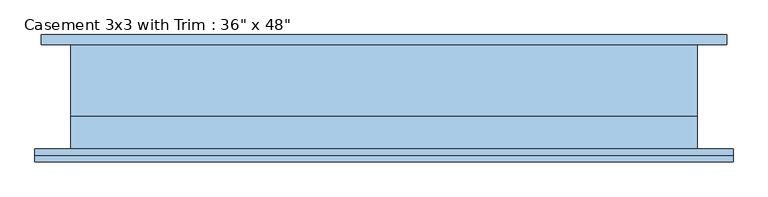
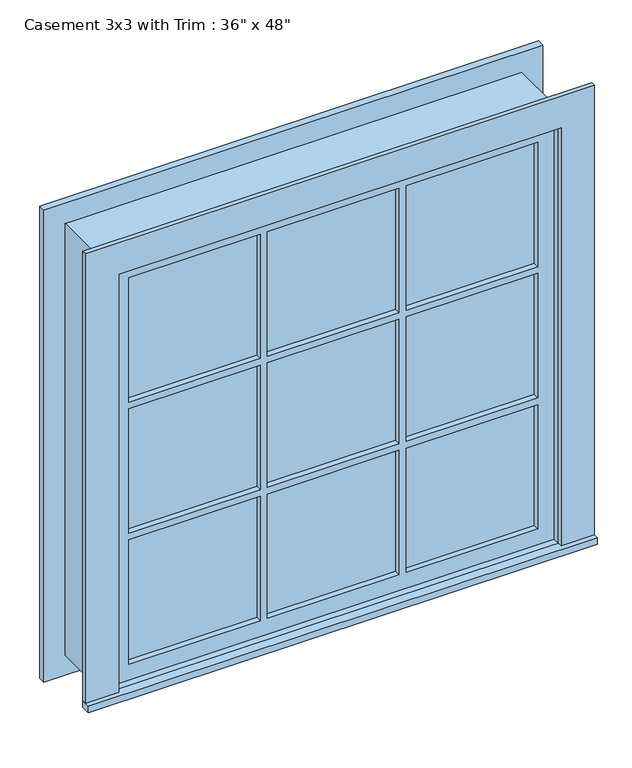
"""IFC4 building model written with IfcOpenShell, lengths in millimetres: window geometry."""

from ifc_helpers import new_model, si_unit, frame, origin, place, context, project, spatial, polyline, outline, extrude, source, transform, mapped, element, save


def window_791d807c(model_context):
    return source(origin(), model_context, "Body", "SweptSolid", [
        extrude(outline(polyline([(-679.45, -127.0), (-679.45, -101.6), (679.45, -101.6), (679.45, -127.0), (-679.45, -127.0)])), frame((0.0, 0.0, 914.4), z_axis=(0.0, 0.0, 1.0), x_axis=(1.0, 0.0, 0.0)), (0.0, 0.0, 1.0), 19.05),
        extrude(outline(polyline([(2114.55, -590.55), (2114.55, 590.55), (933.45, 590.55), (933.45, 679.45), (2203.45, 679.45), (2203.45, -679.45), (933.45, -679.45), (933.45, -590.55), (2114.55, -590.55)])), frame((0.0, -114.3, 0.0), z_axis=(0.0, 1.0, 0.0), x_axis=(0.0, 0.0, 1.0)), (0.0, 0.0, 1.0), 12.7),
        extrude(outline(polyline([(194.7333333, -66.675), (194.7333333, -53.975), (546.1, -53.975), (546.1, -66.675), (194.7333333, -66.675)])), frame((0.0, 0.0, 1718.7333333), z_axis=(0.0, 0.0, 1.0), x_axis=(1.0, 0.0, 0.0)), (0.0, 0.0, 1.0), 351.3666667),
        extrude(outline(polyline([(-175.6833333, -66.675), (-175.6833333, -53.975), (175.6833333, -53.975), (175.6833333, -66.675), (-175.6833333, -66.675)])), frame((0.0, 0.0, 1718.7333333), z_axis=(0.0, 0.0, 1.0), x_axis=(1.0, 0.0, 0.0)), (0.0, 0.0, 1.0), 351.3666667),
        extrude(outline(polyline([(-546.1, -66.675), (-546.1, -53.975), (-194.7333333, -53.975), (-194.7333333, -66.675), (-546.1, -66.675)])), frame((0.0, 0.0, 1718.7333333), z_axis=(0.0, 0.0, 1.0), x_axis=(1.0, 0.0, 0.0)), (0.0, 0.0, 1.0), 351.3666667),
        extrude(outline(polyline([(-546.1, -66.675), (-546.1, -53.975), (-194.7333333, -53.975), (-194.7333333, -66.675), (-546.1, -66.675)])), frame((0.0, 0.0, 1348.3166667), z_axis=(0.0, 0.0, 1.0), x_axis=(1.0, 0.0, 0.0)), (0.0, 0.0, 1.0), 351.3666667),
        extrude(outline(polyline([(-175.6833333, -66.675), (-175.6833333, -53.975), (175.6833333, -53.975), (175.6833333, -66.675), (-175.6833333, -66.675)])), frame((0.0, 0.0, 1348.3166667), z_axis=(0.0, 0.0, 1.0), x_axis=(1.0, 0.0, 0.0)), (0.0, 0.0, 1.0), 351.3666667),
        extrude(outline(polyline([(194.7333333, -66.675), (194.7333333, -53.975), (546.1, -53.975), (546.1, -66.675), (194.7333333, -66.675)])), frame((0.0, 0.0, 1348.3166667), z_axis=(0.0, 0.0, 1.0), x_axis=(1.0, 0.0, 0.0)), (0.0, 0.0, 1.0), 351.3666667),
        extrude(outline(polyline([(194.7333333, -66.675), (194.7333333, -53.975), (546.1, -53.975), (546.1, -66.675), (194.7333333, -66.675)])), frame((0.0, 0.0, 977.9), z_axis=(0.0, 0.0, 1.0), x_axis=(1.0, 0.0, 0.0)), (0.0, 0.0, 1.0), 351.3666667),
        extrude(outline(polyline([(-175.6833333, -66.675), (-175.6833333, -53.975), (175.6833333, -53.975), (175.6833333, -66.675), (-175.6833333, -66.675)])), frame((0.0, 0.0, 977.9), z_axis=(0.0, 0.0, 1.0), x_axis=(1.0, 0.0, 0.0)), (0.0, 0.0, 1.0), 351.3666667),
        extrude(outline(polyline([(-546.1, -66.675), (-546.1, -53.975), (-194.7333333, -53.975), (-194.7333333, -66.675), (-546.1, -66.675)])), frame((0.0, 0.0, 977.9), z_axis=(0.0, 0.0, 1.0), x_axis=(1.0, 0.0, 0.0)), (0.0, 0.0, 1.0), 351.3666667),
        extrude(outline(polyline([(2190.75, 666.75), (2190.75, -666.75), (857.25, -666.75), (857.25, 666.75), (2190.75, 666.75)]), holes=[polyline([(2101.85, 577.85), (946.15, 577.85), (946.15, -577.85), (2101.85, -577.85), (2101.85, 577.85)])]), frame((0.0, 101.6, 0.0), z_axis=(0.0, 1.0, 0.0), x_axis=(0.0, 0.0, 1.0)), (0.0, 0.0, 1.0), 19.05),
        extrude(outline(polyline([(2114.55, -590.55), (933.45, -590.55), (933.45, 590.55), (2114.55, 590.55), (2114.55, -590.55)]), holes=[polyline([(2070.1, -194.7333333), (1718.7333333, -194.7333333), (1718.7333333, -546.1), (2070.1, -546.1), (2070.1, -194.7333333)]), polyline([(1699.6833333, -194.7333333), (1348.3166667, -194.7333333), (1348.3166667, -546.1), (1699.6833333, -546.1), (1699.6833333, -194.7333333)]), polyline([(1329.2666667, -194.7333333), (977.9, -194.7333333), (977.9, -546.1), (1329.2666667, -546.1), (1329.2666667, -194.7333333)]), polyline([(2070.1, 175.6833333), (1718.7333333, 175.6833333), (1718.7333333, -175.6833333), (2070.1, -175.6833333), (2070.1, 175.6833333)]), polyline([(1699.6833333, 175.6833333), (1348.3166667, 175.6833333), (1348.3166667, -175.6833333), (1699.6833333, -175.6833333), (1699.6833333, 175.6833333)]), polyline([(1329.2666667, 175.6833333), (977.9, 175.6833333), (977.9, -175.6833333), (1329.2666667, -175.6833333), (1329.2666667, 175.6833333)]), polyline([(2070.1, 546.1), (1718.7333333, 546.1), (1718.7333333, 194.7333333), (2070.1, 194.7333333), (2070.1, 546.1)]), polyline([(1699.6833333, 546.1), (1348.3166667, 546.1), (1348.3166667, 194.7333333), (1699.6833333, 194.7333333), (1699.6833333, 546.1)]), polyline([(1329.2666667, 546.1), (977.9, 546.1), (977.9, 194.7333333), (1329.2666667, 194.7333333), (1329.2666667, 546.1)])]), frame((0.0, -82.55, 0.0), z_axis=(0.0, 1.0, 0.0), x_axis=(0.0, 0.0, 1.0)), (0.0, 0.0, 1.0), 44.45),
        extrude(outline(polyline([(2133.6, -609.6), (914.4, -609.6), (914.4, 609.6), (2133.6, 609.6), (2133.6, -609.6)]), holes=[polyline([(2101.85, -577.85), (2101.85, 577.85), (946.15, 577.85), (946.15, -577.85), (2101.85, -577.85)])]), frame((0.0, -38.1, 0.0), z_axis=(0.0, 1.0, 0.0), x_axis=(0.0, 0.0, 1.0)), (0.0, 0.0, 1.0), 139.7),
        extrude(outline(polyline([(2133.6, 609.6), (2133.6, -609.6), (914.4, -609.6), (914.4, 609.6), (2133.6, 609.6)]), holes=[polyline([(2114.55, 590.55), (933.45, 590.55), (933.45, -590.55), (2114.55, -590.55), (2114.55, 590.55)])]), frame((0.0, -101.6, 0.0), z_axis=(0.0, 1.0, 0.0), x_axis=(0.0, 0.0, 1.0)), (0.0, 0.0, 1.0), 63.5),
    ])


if __name__ == "__main__":
    model = new_model("IFC4")
    model_context = context("Model", 3, world=origin())
    ifc_project = project(units=[si_unit("LENGTHUNIT", "METRE", prefix="MILLI")], contexts=[model_context])
    site = spatial("IfcSite", under=ifc_project)
    building = spatial("IfcBuilding", under=site)
    placement = place(None, origin())
    window_shape = window_791d807c(model_context)
    element("IfcWindow", 1, ObjectType="Casement 3x3 with Trim : 36\" x 48\"", at=placement, inside=building, context=model_context, shape_type="MappedRepresentation", body=[
        mapped(window_shape, transform((0.0, 0.0, 0.0), x_axis=(1.0, 0.0, 0.0), y_axis=(0.0, 1.0, 0.0), z_axis=(0.0, 0.0, 1.0))),
    ])
    save(model, "model.ifc")

# Revit data of these elements
# Type "Casement 3x3 with Trim : 36\" x 48\""
#   Type Mark = "10"
#   Construction Type Id = "GSP4R"
#   Assembly Code = "B2020100"
#   Analytic Construction = "1/8 in Pilkington single glazing"
#   Visual Light Transmittance = 0.9
#   Solar Heat Gain Coefficient = 0.78
#   Heat Transfer Coefficient (U) = 0.6496 BTU/(h·ft²·°F)
#   Height = 4' - 0"
#   Default Sill Height = 3' - 0"
#   Trim Projection - Ext. = 0' - 0 1/2"
#   Trim Projection - Int. = 0' - 0 3/4"
#   Trim Width - Exterior = 0' - 3 1/2"
#   Trim Width - Interior = 0' - 3 1/2"
#   Width = 4' - 0"
#   Window Inset = 0' - 0 3/4"
#   Define Thermal Properties by = 1
#   Glass Pane Material = Glass
#   Sash Material = Sash
#   Trim Exterior Material = Trim
#   Trim Interior Material = Trim
#   Wall Closure = (empty or 0)
# Element 1 (IfcWindow, "Casement 3x3 with Trim : 36\" x 48\"")
#   Materials on its faces: "Sash", "Glass", "Trim"
# Materials
#   "Glass": class "Glass", colour RGB 0 128 192, transparency 0.75, Description = "Soda Lime Glass", Cost = 0
#   "Sash": class "Wood", colour RGB 224 178 126, transparency 0
#   "Trim": class "Wood", colour RGB 224 178 126, transparency 0
